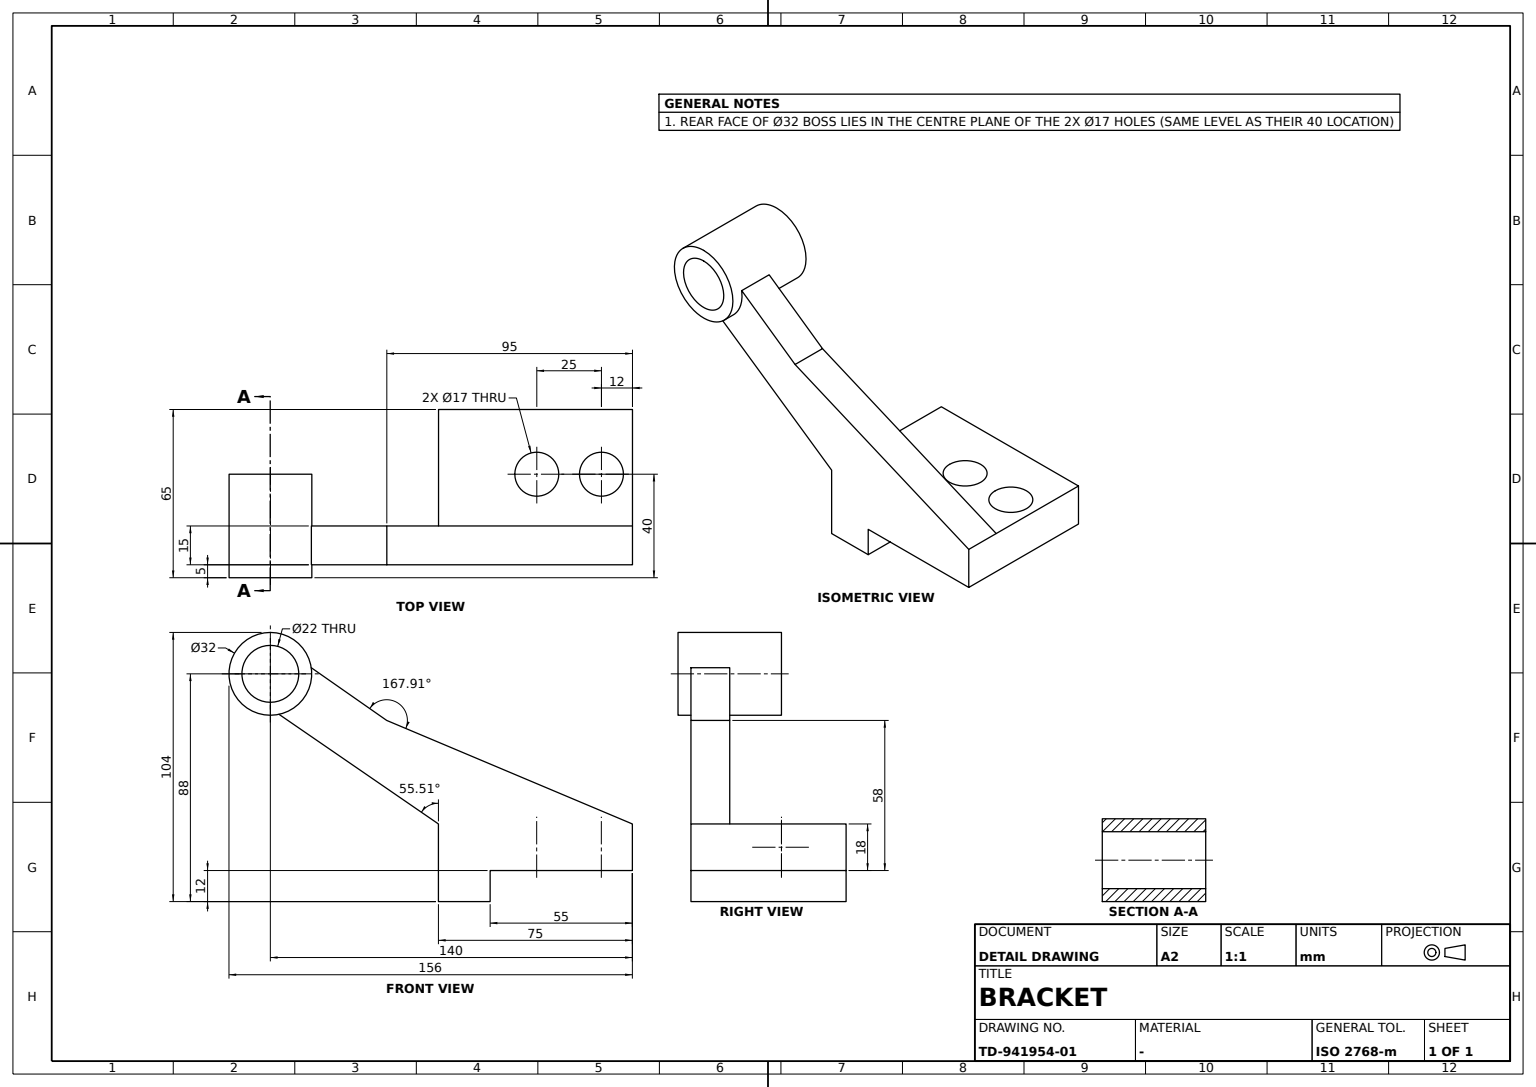
CATIA V5 part; units mm, degrees
sketch "Sketch1" plane through (0, 0, 0) normal (0, 1, 0) x (-1, 0, 0)
  line L0 (0, 0) -> (0, 18)
  line L1 (0, 18) -> (75, 18)
  line L2 (75, 18) -> (75, -12)
  line L3 (75, -12) -> (55, -12)
  line L4 (55, -12) -> (55, 0)
  point P0 (55, 0)
  line L5 (55, 0) -> (0, 0)
  dimension "length L5" = 55
  dimension "distance L0 L2" = 75
  dimension "length L0" = 18
  dimension "length L2" = 30
  constraint vertical L0 y-axis
  constraint vertical L2 y-axis
  constraint vertical L4 y-axis
  constraint horizontal L1 x-axis
  constraint horizontal L3 x-axis
  constraint horizontal L5 x-axis
  constraint coincidence P0 x-axis
extrude "Pad1" add sketch "Sketch1" along normal blind 60
sketch "Sketch2" plane through (0, 0, 0) normal (0, 1, 0) x (-1, 0, 0)
  point P0 (140, 76)
  line L0 (0, 18) -> (95, 58)
  point P1 (0, 18)
  point P2 (95, 58)
  line L1 (75, 18) -> (0, 18) construction
  line L2 (75, 18) -> (0, 18)
  point P3 (0, 18)
  arc A0 (146.2287, 66.9334) -> (133.7033, 85.0195) centre (140, 76) ccw
  line L3 (55, -12) -> (75, -12) construction
  line L4 (95, 58) -> (133.7033, 85.0195)
  line L5 (75, 18) -> (146.2287, 66.9334)
  dimension "distance y axis P0" = 140
  dimension "distance y axis P2" = 95
  dimension "distance P2 x axis" = 58
  dimension "radius A0" = 11
  dimension "distance L3 P0" = 88
  constraint coincidence P1 y-axis
  constraint coincidence P1 L1
  constraint coincidence P1 P3
  constraint tangency L4 A0
  constraint tangency L5 A0
extrude "Pad2" add sketch "Sketch2" along normal blind 15
sketch "Sketch4" plane through (0, 0, 0) normal (0, 1, 0) x (-1, 0, 0)
  circle A0 centre (140, 76) radius 16
  arc A1 (146.2287, 66.9334) -> (133.7033, 85.0195) centre (140, 76) ccw construction
  dimension "radius A0" = 16
  constraint concentricity A0 A1
extrude "Pad3" add sketch "Sketch4" along normal blind 15
sketch "Sketch5" plane through (0, 0, 0) normal (0, 1, 0) x (-1, 0, 0)
  circle A0 centre (140, 76) radius 11
  circle A1 centre (140, 76) radius 16 construction
  dimension "radius A0" = 11
  constraint concentricity A0 A1
extrude "Pocket1" cut sketch "Sketch5" along normal blind 15
sketch "Sketch6" plane through (0, 0, 0) normal (0, 1, 0) x (-1, 0, 0)
  circle A0 centre (140, 76) radius 16
  circle A1 centre (140, 76) radius 16 construction
  circle A2 centre (140, 76) radius 11
  dimension "radius A0" = 16
  constraint concentricity A0 A1
extrude "Pad4" add sketch "Sketch6" against normal blind 5
sketch "Sketch7" plane through (0, 15, 0) normal (0, 1, 0) x (-1, 0, 0)
  circle A0 centre (140, 76) radius 16
  circle A1 centre (140, 76) radius 16 construction
  circle A2 centre (140, 76) radius 11
  dimension "radius A0" = 16
  constraint concentricity A0 A1
extrude "Pad5" add sketch "Sketch7" against normal blind 5
sketch "Sketch3" plane through (0, 15, 0) normal (0, 1, 0) x (-1, 0, 0)
  circle A0 centre (140, 76) radius 16
  circle A1 centre (140, 76) radius 16 construction
  circle A2 centre (140, 76) radius 11
  dimension "radius A0" = 16
  constraint concentricity A0 A1
extrude "Pad6" add sketch "Sketch3" along normal blind 20
sketch "Sketch8" plane through (0, 0, 0) normal (0, 0, 1) x (1, 0, 0)
  circle A0 centre (-37, 35) radius 8.5
  point P0 (-37, 35)
  circle A1 centre (-12, 35) radius 8.5
  point P1 (-12, 35)
  line L0 (-75, 60) -> (0, 60) construction
  line L1 (-75, 60) -> (0, 60) construction
  dimension "radius A1" = 8.5
  dimension "radius A0" = 8.5
  dimension "distance P1 y axis" = 12
  dimension "distance P0 P1" = 25
  dimension "distance P0 L0" = 25
  dimension "distance P1 L1" = 25
extrude "Pocket2" cut sketch "Sketch8" along normal blind 20
properties part number "1"
